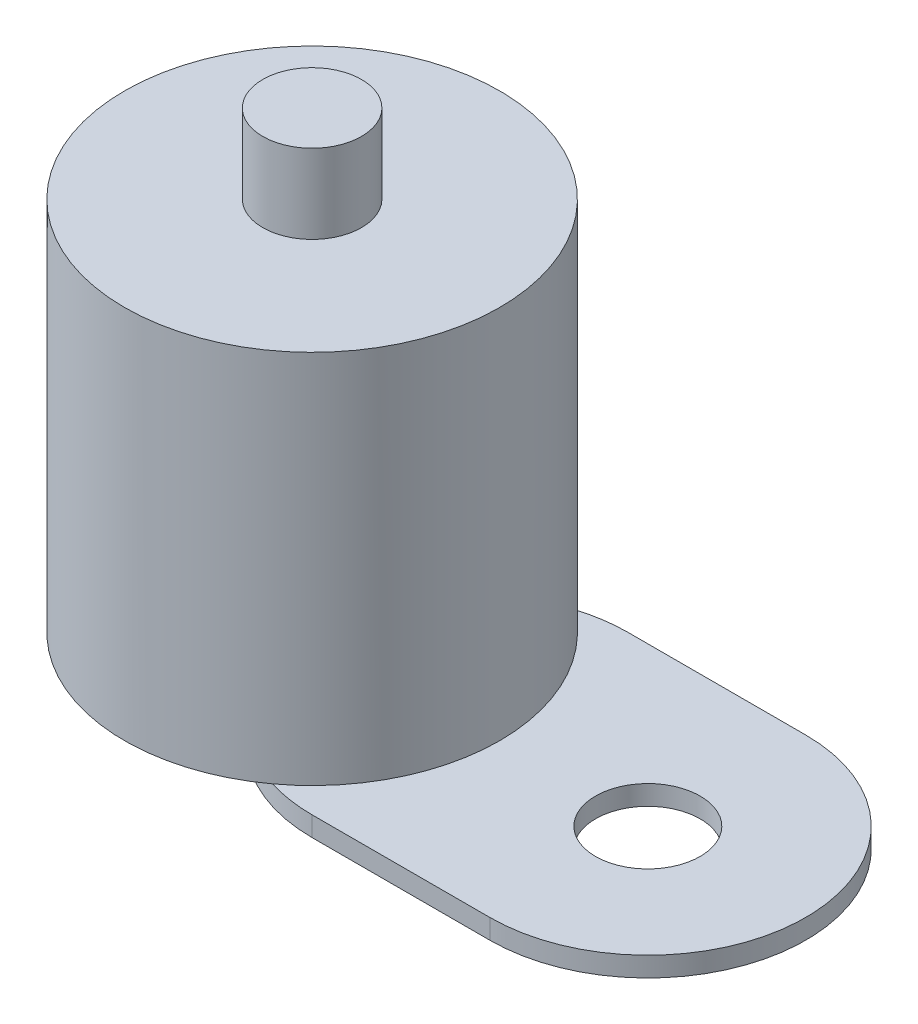
SolidWorks part; units mm, degrees
material "Plain Carbon Steel"
ref_plane "Front Plane" through (0, 0, 0) normal (0, 0, 1) x (1, 0, 0)
ref_plane "Top Plane" through (0, 0, 0) normal (0, 1, 0) x (1, 0, 0)
ref_plane "Right Plane" through (0, 0, 0) normal (1, 0, 0) x (0, 0, -1)
sketch "Mounting Tab Profile" plane through (0, 0, 0) normal (0, 1, 0) x (1, 0, 0)
  line L0 (-4.5, 0) -> (4.5, 0) construction
  line L1 (-4.5, 8) -> (4.5, 8)
  line L2 (-4.5, -8) -> (4.5, -8)
  line L3 (-12.5, 0) -> (-12.5, -8.9832) construction
  arc A0 (-4.5, 8) -> (-4.5, -8) centre (-4.5, 0) ccw
  arc A1 (4.5, -8) -> (4.5, 8) centre (4.5, 0) ccw
  circle A2 centre (4.5, 0) radius 2.65
  point P2 (0, 0)
  point P10 (12.5, 0)
  dimension "D1" = 25
  dimension "8" = 8
  dimension "D2" = 5.3
extrude "Mounting Tab 1mm with Hole Ø5.3" add sketch "Mounting Tab Profile" along normal blind 1
sketch "Chamber Body Profile Ø19" plane through (0, 1, 0) normal (0, 1, 0) x (1, 0, 0)
  line L0 (14.6582, 0) -> (-25.9374, 0) construction
  circle A0 centre (-12.5, 0) radius 9.5
  arc A1 (-4.5, 8) -> (-4.5, -8) centre (-4.5, 0) ccw construction
  dimension "D1" = 19
extrude "Chamber Body Ø19x19" add sketch "Chamber Body Profile Ø19" along normal blind 19
sketch "Top Pin Profile Ø5" plane through (0, 20, 0) normal (0, 1, 0) x (1, 0, 0)
  circle A0 centre (-12.5, 0) radius 2.5
  dimension "D1" = 5
extrude "Top Pin Ø5x4" add sketch "Top Pin Profile Ø5" along normal blind 4
